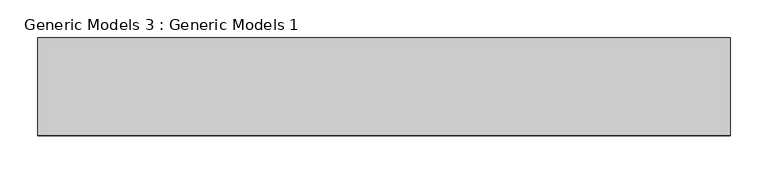
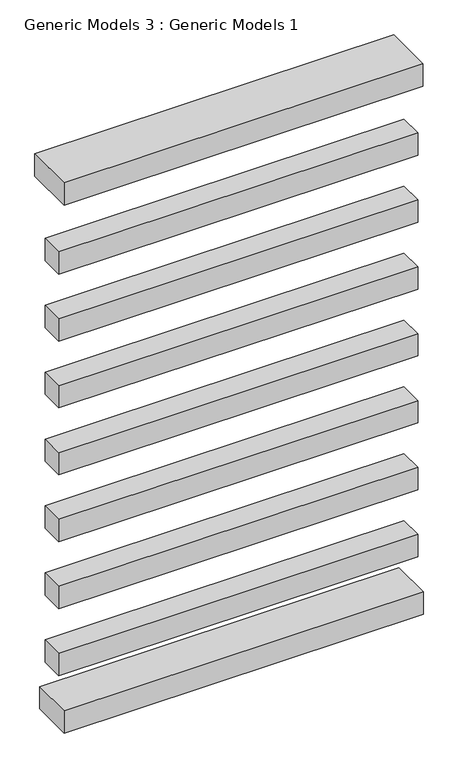
"""IFC4 building model written with IfcOpenShell, lengths in millimetres: proxy geometry, Generic Models 3 : Generic Models 1."""

from ifc_helpers import new_model, si_unit, origin, place, context, project, spatial, faceted_brep, source, transform, mapped, element, save


def generic_models_3_generic_models_1_2aceec8a(model_context):
    return source(origin(), model_context, "Body", "Brep", [
        faceted_brep([(-2400.2544048, -6113.8685722, -385.6320944), (-2400.2544048, -6113.8685722, -445.6320944), (-2400.2544048, -6221.5933823, -445.6320944), (-2400.2544048, -6221.5933823, -385.6320944), (-1485.8544048, -6113.8685722, -385.6320944), (-1485.8544048, -6221.5933823, -385.6320944), (-1485.8544048, -6221.5933823, -445.6320944), (-1485.8544048, -6113.8685722, -445.6320944), (-2269.6353385, -6113.8685722, -385.6320944), (-2392.6544048, -6113.8685722, -385.6320944), (-2392.6544048, -6113.8685722, -445.6320944), (-2269.6353385, -6113.8685722, -445.6320944)], [[[0, 1, 2, 3]], [[4, 5, 6, 7]], [[0, 3, 5, 4, 8, 9]], [[3, 2, 6, 5]], [[2, 1, 10, 11, 7, 6]], [[1, 0, 9, 8, 4, 7, 11, 10]]]),
        faceted_brep([(-2400.2544048, -6137.2837816, -245.6320944), (-2400.2544048, -6137.2837816, -305.6320944), (-2400.2544048, -6197.2837816, -305.6320944), (-2400.2544048, -6197.2837816, -245.6320944), (-1485.8544048, -6137.2837816, -245.6320944), (-1485.8544048, -6197.2837816, -245.6320944), (-1485.8544048, -6197.2837816, -305.6320944), (-1485.8544048, -6137.2837816, -305.6320944), (-2392.6544048, -6197.2837816, -245.6320944), (-2269.6353385, -6197.2837816, -245.6320944), (-2269.6353385, -6137.2837816, -245.6320944), (-2392.6544048, -6137.2837816, -245.6320944), (-2392.6544048, -6197.2837816, -305.6320944), (-2269.6353385, -6197.2837816, -305.6320944), (-2392.6544048, -6137.2837816, -305.6320944), (-2269.6353385, -6137.2837816, -305.6320944)], [[[0, 1, 2, 3]], [[4, 5, 6, 7]], [[0, 3, 8, 9, 5, 4, 10, 11]], [[3, 2, 12, 13, 6, 5, 9, 8]], [[2, 1, 14, 15, 7, 6, 13, 12]], [[1, 0, 11, 10, 4, 7, 15, 14]]]),
        faceted_brep([(-2400.2544048, -6137.2837816, -65.6320944), (-2400.2544048, -6137.2837816, -125.6320944), (-2400.2544048, -6197.2837816, -125.6320944), (-2400.2544048, -6197.2837816, -65.6320944), (-1485.8544048, -6137.2837816, -65.6320944), (-1485.8544048, -6197.2837816, -65.6320944), (-1485.8544048, -6197.2837816, -125.6320944), (-1485.8544048, -6137.2837816, -125.6320944), (-2392.6544048, -6197.2837816, -65.6320944), (-2269.6353385, -6197.2837816, -65.6320944), (-2269.6353385, -6137.2837816, -65.6320944), (-2392.6544048, -6137.2837816, -65.6320944), (-2392.6544048, -6197.2837816, -125.6320944), (-2269.6353385, -6197.2837816, -125.6320944), (-2392.6544048, -6137.2837816, -125.6320944), (-2269.6353385, -6137.2837816, -125.6320944)], [[[0, 1, 2, 3]], [[4, 5, 6, 7]], [[0, 3, 8, 9, 5, 4, 10, 11]], [[3, 2, 12, 13, 6, 5, 9, 8]], [[2, 1, 14, 15, 7, 6, 13, 12]], [[1, 0, 11, 10, 4, 7, 15, 14]]]),
        faceted_brep([(-2400.2544048, -6137.2837816, 114.3679056), (-2400.2544048, -6137.2837816, 54.3679056), (-2400.2544048, -6197.2837816, 54.3679056), (-2400.2544048, -6197.2837816, 114.3679056), (-1485.8544048, -6137.2837816, 114.3679056), (-1485.8544048, -6197.2837816, 114.3679056), (-1485.8544048, -6197.2837816, 54.3679056), (-1485.8544048, -6137.2837816, 54.3679056), (-2392.6544048, -6197.2837816, 114.3679056), (-2269.6353385, -6197.2837816, 114.3679056), (-2269.6353385, -6137.2837816, 114.3679056), (-2392.6544048, -6137.2837816, 114.3679056), (-2392.6544048, -6197.2837816, 54.3679056), (-2269.6353385, -6197.2837816, 54.3679056), (-2392.6544048, -6137.2837816, 54.3679056), (-2269.6353385, -6137.2837816, 54.3679056)], [[[0, 1, 2, 3]], [[4, 5, 6, 7]], [[0, 3, 8, 9, 5, 4, 10, 11]], [[3, 2, 12, 13, 6, 5, 9, 8]], [[2, 1, 14, 15, 7, 6, 13, 12]], [[1, 0, 11, 10, 4, 7, 15, 14]]]),
        faceted_brep([(-2400.2544048, -6137.2837816, 294.3679056), (-2400.2544048, -6137.2837816, 234.3679056), (-2400.2544048, -6197.2837816, 234.3679056), (-2400.2544048, -6197.2837816, 294.3679056), (-1485.8544048, -6137.2837816, 294.3679056), (-1485.8544048, -6197.2837816, 294.3679056), (-1485.8544048, -6197.2837816, 234.3679056), (-1485.8544048, -6137.2837816, 234.3679056), (-2392.6544048, -6197.2837816, 294.3679056), (-2269.6353385, -6197.2837816, 294.3679056), (-2269.6353385, -6137.2837816, 294.3679056), (-2392.6544048, -6137.2837816, 294.3679056), (-2392.6544048, -6197.2837816, 234.3679056), (-2269.6353385, -6197.2837816, 234.3679056), (-2392.6544048, -6137.2837816, 234.3679056), (-2269.6353385, -6137.2837816, 234.3679056)], [[[0, 1, 2, 3]], [[4, 5, 6, 7]], [[0, 3, 8, 9, 5, 4, 10, 11]], [[3, 2, 12, 13, 6, 5, 9, 8]], [[2, 1, 14, 15, 7, 6, 13, 12]], [[1, 0, 11, 10, 4, 7, 15, 14]]]),
        faceted_brep([(-2400.2544048, -6137.2837816, 474.3679056), (-2400.2544048, -6137.2837816, 414.3679056), (-2400.2544048, -6197.2837816, 414.3679056), (-2400.2544048, -6197.2837816, 474.3679056), (-1485.8544048, -6137.2837816, 474.3679056), (-1485.8544048, -6197.2837816, 474.3679056), (-1485.8544048, -6197.2837816, 414.3679056), (-1485.8544048, -6137.2837816, 414.3679056), (-2392.6544048, -6197.2837816, 474.3679056), (-2269.6353385, -6197.2837816, 474.3679056), (-2269.6353385, -6137.2837816, 474.3679056), (-2392.6544048, -6137.2837816, 474.3679056), (-2392.6544048, -6197.2837816, 414.3679056), (-2269.6353385, -6197.2837816, 414.3679056), (-2392.6544048, -6137.2837816, 414.3679056), (-2269.6353385, -6137.2837816, 414.3679056)], [[[0, 1, 2, 3]], [[4, 5, 6, 7]], [[0, 3, 8, 9, 5, 4, 10, 11]], [[3, 2, 12, 13, 6, 5, 9, 8]], [[2, 1, 14, 15, 7, 6, 13, 12]], [[1, 0, 11, 10, 4, 7, 15, 14]]]),
        faceted_brep([(-2400.2544048, -6137.2837816, 654.3679056), (-2400.2544048, -6137.2837816, 594.3679056), (-2400.2544048, -6197.2837816, 594.3679056), (-2400.2544048, -6197.2837816, 654.3679056), (-1485.8544048, -6137.2837816, 654.3679056), (-1485.8544048, -6197.2837816, 654.3679056), (-1485.8544048, -6197.2837816, 594.3679056), (-1485.8544048, -6137.2837816, 594.3679056), (-2392.6544048, -6197.2837816, 654.3679056), (-2269.6353385, -6197.2837816, 654.3679056), (-2269.6353385, -6137.2837816, 654.3679056), (-2392.6544048, -6137.2837816, 654.3679056), (-2392.6544048, -6197.2837816, 594.3679056), (-2269.6353385, -6197.2837816, 594.3679056), (-2392.6544048, -6137.2837816, 594.3679056), (-2269.6353385, -6137.2837816, 594.3679056)], [[[0, 1, 2, 3]], [[4, 5, 6, 7]], [[0, 3, 8, 9, 5, 4, 10, 11]], [[3, 2, 12, 13, 6, 5, 9, 8]], [[2, 1, 14, 15, 7, 6, 13, 12]], [[1, 0, 11, 10, 4, 7, 15, 14]]]),
        faceted_brep([(-2400.2544048, -6137.2837816, 834.3679056), (-2400.2544048, -6137.2837816, 774.3679056), (-2400.2544048, -6197.2837816, 774.3679056), (-2400.2544048, -6197.2837816, 834.3679056), (-1485.8544048, -6137.2837816, 834.3679056), (-1485.8544048, -6197.2837816, 834.3679056), (-1485.8544048, -6197.2837816, 774.3679056), (-1485.8544048, -6137.2837816, 774.3679056), (-2392.6544048, -6197.2837816, 834.3679056), (-2269.6353385, -6197.2837816, 834.3679056), (-2269.6353385, -6137.2837816, 834.3679056), (-2392.6544048, -6137.2837816, 834.3679056), (-2392.6544048, -6197.2837816, 774.3679056), (-2269.6353385, -6197.2837816, 774.3679056), (-2392.6544048, -6137.2837816, 774.3679056), (-2269.6353385, -6137.2837816, 774.3679056)], [[[0, 1, 2, 3]], [[4, 5, 6, 7]], [[0, 3, 8, 9, 5, 4, 10, 11]], [[3, 2, 12, 13, 6, 5, 9, 8]], [[2, 1, 14, 15, 7, 6, 13, 12]], [[1, 0, 11, 10, 4, 7, 15, 14]]]),
        faceted_brep([(-2400.2544048, -6092.2648653, 1034.3679056), (-2400.2544048, -6092.2648653, 974.3679056), (-2400.2544048, -6220.9896754, 974.3679056), (-2400.2544048, -6220.9896754, 1034.3679056), (-1485.8544048, -6092.2648653, 1034.3679056), (-1485.8544048, -6220.9896754, 1034.3679056), (-1485.8544048, -6220.9896754, 974.3679056), (-1485.8544048, -6092.2648653, 974.3679056), (-2392.6544048, -6220.9896754, 974.3679056), (-2269.6353385, -6220.9896754, 974.3679056), (-2392.6544048, -6092.2648653, 974.3679056), (-2269.6353385, -6092.2648653, 974.3679056)], [[[0, 1, 2, 3]], [[4, 5, 6, 7]], [[0, 3, 5, 4]], [[3, 2, 8, 9, 6, 5]], [[2, 1, 10, 11, 7, 6, 9, 8]], [[1, 0, 4, 7, 11, 10]]]),
    ])


if __name__ == "__main__":
    model = new_model("IFC4")
    model_context = context("Model", 3, world=origin())
    ifc_project = project(units=[si_unit("LENGTHUNIT", "METRE", prefix="MILLI")], contexts=[model_context])
    site = spatial("IfcSite", under=ifc_project)
    building = spatial("IfcBuilding", under=site)
    placement = place(None, origin())
    generic_models_3_generic_models_1_shape = generic_models_3_generic_models_1_2aceec8a(model_context)
    element("IfcBuildingElementProxy", 1, Name="Generic Models 3 : Generic Models 1", ObjectType="Generic Models 3 : Generic Models 1", at=placement, inside=building, context=model_context, shape_type="MappedRepresentation", body=[
        mapped(generic_models_3_generic_models_1_shape, transform((0.0, 0.0, 0.0), x_axis=(1.0, 0.0, 0.0), y_axis=(0.0, 1.0, 0.0), z_axis=(0.0, 0.0, 1.0))),
    ])
    save(model, "model.ifc")
